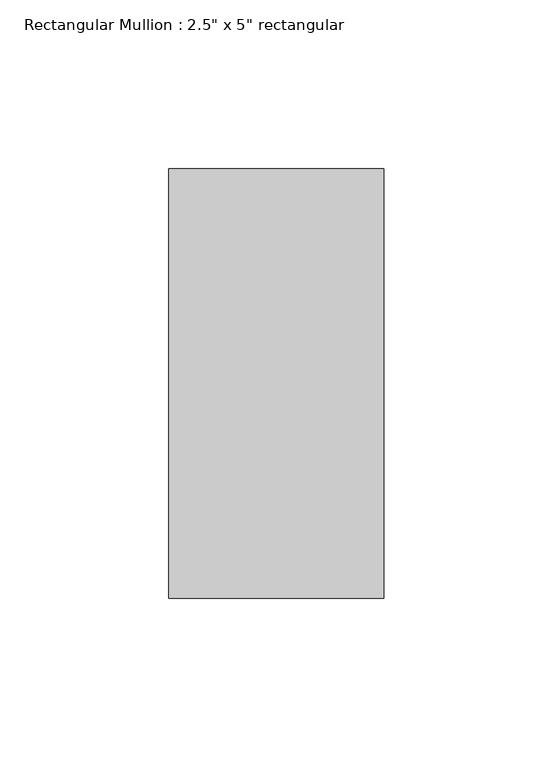
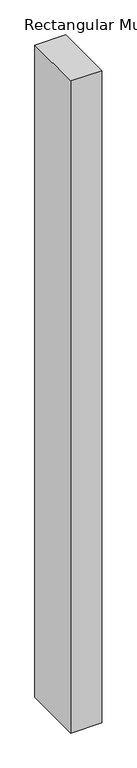
"""IFC4 building model written with IfcOpenShell, lengths in millimetres: member geometry."""

from ifc_helpers import new_model, si_unit, frame, origin, place, context, project, spatial, polyline, outline, extrude, source, transform, mapped, element, save


def member_0dc43c0c(model_context):
    return source(origin(), model_context, "Body", "SweptSolid", [
        extrude(outline(polyline([(0.0, 63.5), (0.0, -63.5), (-63.5, -63.5), (-63.5, 63.5), (0.0, 63.5)])), frame((0.0, 0.0, -1409.6999998), z_axis=(0.0, 0.0, 1.0), x_axis=(1.0, 0.0, 0.0)), (0.0, 0.0, 1.0), 1409.6999998),
    ])


if __name__ == "__main__":
    model = new_model("IFC4")
    model_context = context("Model", 3, world=origin())
    ifc_project = project(units=[si_unit("LENGTHUNIT", "METRE", prefix="MILLI")], contexts=[model_context])
    site = spatial("IfcSite", under=ifc_project)
    building = spatial("IfcBuilding", under=site)
    placement = place(None, origin())
    member_shape = member_0dc43c0c(model_context)
    element("IfcMember", 1, ObjectType="Rectangular Mullion : 2.5\" x 5\" rectangular", at=placement, inside=building, context=model_context, shape_type="MappedRepresentation", body=[
        mapped(member_shape, transform((0.0, 0.0, 0.0), x_axis=(1.0, 0.0, 0.0), y_axis=(0.0, 1.0, 0.0), z_axis=(0.0, 0.0, 1.0))),
    ])
    save(model, "model.ifc")

# Revit data of these elements
# Type "Rectangular Mullion : 2.5\" x 5\" rectangular"
#   built-in parameter 1007304 = 0.416667 (stored number, unit not read)
#   built-in parameter 1007301 = 0.104167 (stored number, unit not read)
#   built-in parameter 1007300 = 0.104167 (stored number, unit not read)
# Element 1 (IfcMember, "Rectangular Mullion : 2.5\" x 5\" rectangular")
#   Materials on its faces: "WINDOW FRAMING"
# Materials
#   "WINDOW FRAMING": class "Generic", colour RGB 120 120 120, transparency 0, Cost = 0
